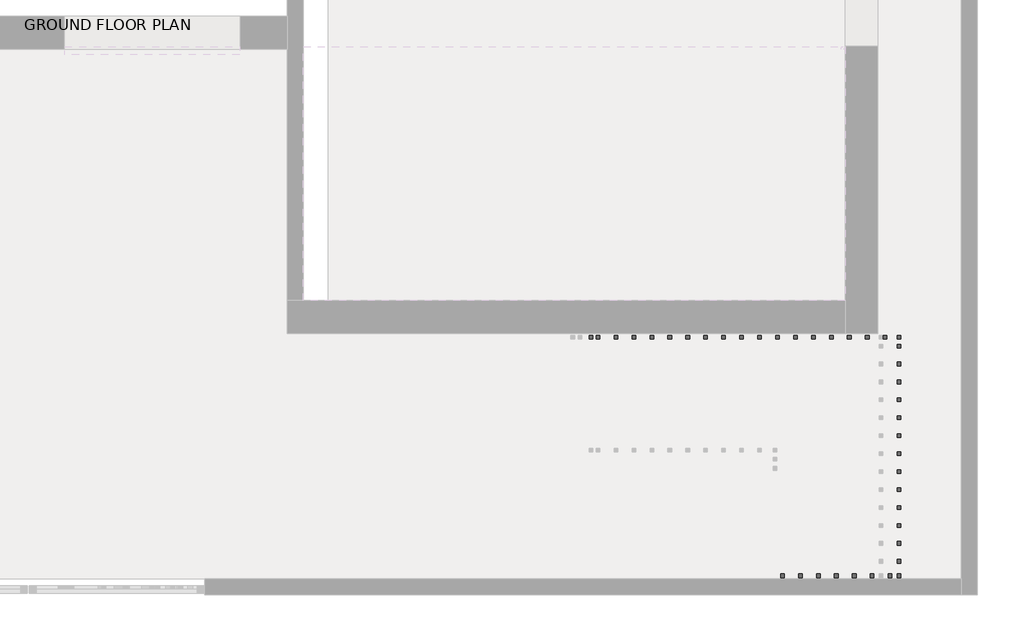
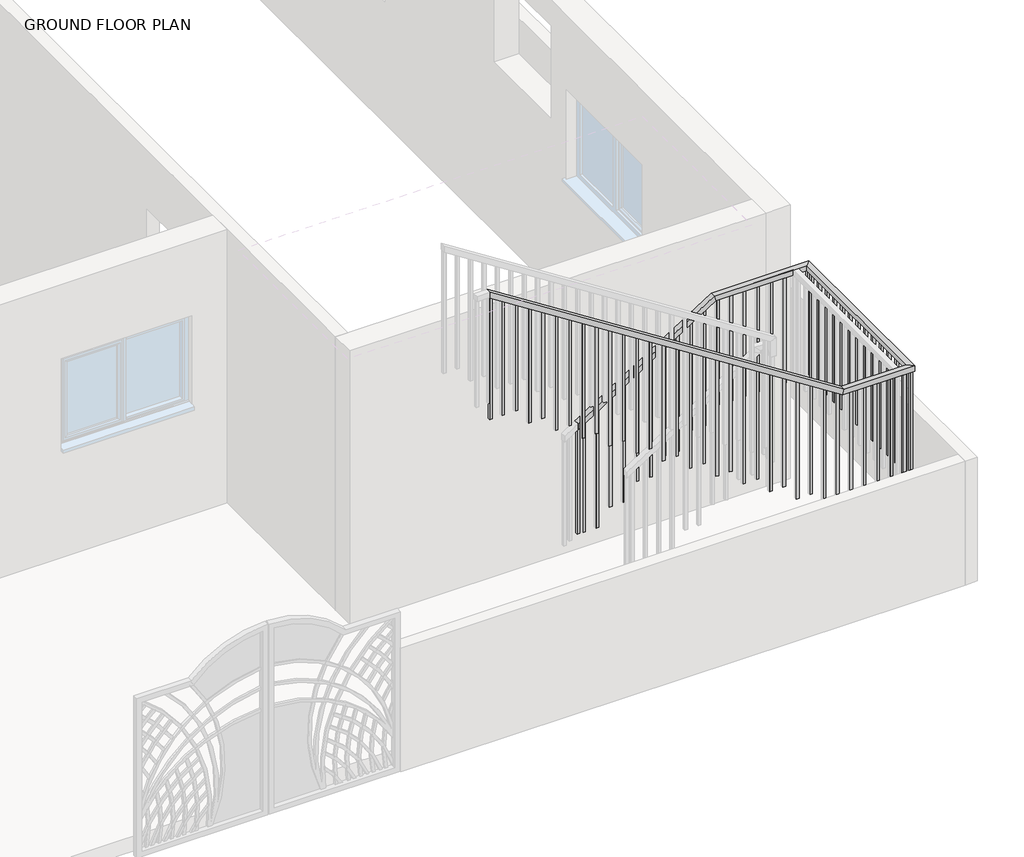
# One storey, part 2 of 23: 2 railings.
"""IFC4 building model written with IfcOpenShell, lengths in millimetres."""

from ifc_helpers import new_model, si_unit, frame, origin, place, context, project, spatial, polyline, outline, extrude, faceted_brep, element, save

model = new_model("IFC4")

# Units and contexts
model_context = context("Model", 3, world=origin())
ifc_project = project(units=[si_unit("LENGTHUNIT", "METRE", prefix="MILLI")], contexts=[model_context])

# Site, building, storey
site = spatial("IfcSite", under=ifc_project)
building = spatial("IfcBuilding", under=site)
storey = spatial("IfcBuildingStorey", under=building, Name="GROUND FLOOR PLAN", Elevation=487.68)

# Railings
placement = place(None, origin())
element("IfcRailing", 1, ObjectType="1100mm", at=placement, inside=storey, context=model_context, shape_type="SolidModel", body=[
    faceted_brep([(-8680.149573, -10220.0521308, 1912.8), (-8680.149573, -10220.0521308, 1853.4423995), (-8680.149573, -10270.0521308, 1853.4423995), (-8680.149573, -10270.0521308, 1912.8), (-7409.7306254, -10220.0521308, 2725.6), (-7395.1045513, -10220.0521308, 2675.6), (-7395.1045513, -10270.0521308, 2675.6), (-7409.7306254, -10270.0521308, 2725.6), (-6495.8132565, -10220.0521308, 2725.6), (-6495.8132565, -10220.0521308, 2675.6), (-6545.8132565, -10270.0521308, 2675.6), (-6545.8132565, -10270.0521308, 2725.6), (-6495.8132565, -11933.6860066, 2725.6), (-6495.8132565, -11933.6860066, 2675.6), (-6545.8132565, -11883.6860066, 2675.6), (-6545.8132565, -11883.6860066, 2725.6), (-7155.718398, -11933.6860066, 2725.6), (-7170.3479429, -11933.6860066, 2675.6), (-7170.3479429, -11883.6860066, 2675.6), (-7155.718398, -11883.6860066, 2725.6), (-10457.8773536, -11933.6860066, 4838.88), (-10457.8773536, -11883.6860066, 4838.88), (-10457.8773536, -11883.6860066, 4779.517542), (-10457.8773536, -11933.6860066, 4779.517542)], [[[0, 1, 2, 3]], [[1, 0, 4, 5]], [[2, 1, 5, 6]], [[3, 2, 6, 7]], [[0, 3, 7, 4]], [[5, 4, 8, 9]], [[6, 5, 9, 10]], [[7, 6, 10, 11]], [[4, 7, 11, 8]], [[9, 8, 12, 13]], [[10, 9, 13, 14]], [[11, 10, 14, 15]], [[8, 11, 15, 12]], [[13, 12, 16, 17]], [[14, 13, 17, 18]], [[15, 14, 18, 19]], [[12, 15, 19, 16]], [[20, 21, 22, 23]], [[17, 16, 20, 23]], [[18, 17, 23, 22]], [[19, 18, 22, 21]], [[16, 19, 21, 20]]]),
    extrude(outline(polyline([(4691.8007425, -10320.8132565), (4707.7999723, -10345.8132565), (3576.32, -10345.8132565), (3576.32, -10320.8132565), (4691.8007425, -10320.8132565)])), frame((0.0, -11921.1860066, 0.0), z_axis=(0.0, 1.0, 0.0), x_axis=(0.0, 0.0, 1.0)), (0.0, 0.0, 1.0), 25.0),
    extrude(outline(polyline([(4611.8045935, -10195.8132565), (4627.8038233, -10220.8132565), (3576.32, -10220.8132565), (3576.32, -10195.8132565), (4611.8045935, -10195.8132565)])), frame((0.0, -11921.1860066, 0.0), z_axis=(0.0, 1.0, 0.0), x_axis=(0.0, 0.0, 1.0)), (0.0, 0.0, 1.0), 25.0),
    extrude(outline(polyline([(4531.8084444, -10070.8132565), (4547.8076742, -10095.8132565), (3413.76, -10095.8132565), (3413.76, -10070.8132565), (4531.8084444, -10070.8132565)])), frame((0.0, -11921.1860066, 0.0), z_axis=(0.0, 1.0, 0.0), x_axis=(0.0, 0.0, 1.0)), (0.0, 0.0, 1.0), 25.0),
    extrude(outline(polyline([(4451.8122954, -9945.8132565), (4467.8115252, -9970.8132565), (3413.76, -9970.8132565), (3413.76, -9945.8132565), (4451.8122954, -9945.8132565)])), frame((0.0, -11921.1860066, 0.0), z_axis=(0.0, 1.0, 0.0), x_axis=(0.0, 0.0, 1.0)), (0.0, 0.0, 1.0), 25.0),
    extrude(outline(polyline([(4371.8161463, -9820.8132565), (4387.8153761, -9845.8132565), (3251.2, -9845.8132565), (3251.2, -9820.8132565), (4371.8161463, -9820.8132565)])), frame((0.0, -11921.1860066, 0.0), z_axis=(0.0, 1.0, 0.0), x_axis=(0.0, 0.0, 1.0)), (0.0, 0.0, 1.0), 25.0),
    extrude(outline(polyline([(4291.8423995, -9695.8132565), (4307.8371231, -9720.8132565), (3251.2, -9720.8132565), (3251.2, -9695.8132565), (4291.8423995, -9695.8132565)])), frame((0.0, -11921.1860066, 0.0), z_axis=(0.0, 1.0, 0.0), x_axis=(0.0, 0.0, 1.0)), (0.0, 0.0, 1.0), 25.0),
    extrude(outline(polyline([(4211.8238482, -9570.8132565), (4227.823078, -9595.8132565), (3088.64, -9595.8132565), (3088.64, -9570.8132565), (4211.8238482, -9570.8132565)])), frame((0.0, -11921.1860066, 0.0), z_axis=(0.0, 1.0, 0.0), x_axis=(0.0, 0.0, 1.0)), (0.0, 0.0, 1.0), 25.0),
    extrude(outline(polyline([(4131.8276992, -9445.8132565), (4147.826929, -9470.8132565), (3088.64, -9470.8132565), (3088.64, -9445.8132565), (4131.8276992, -9445.8132565)])), frame((0.0, -11921.1860066, 0.0), z_axis=(0.0, 1.0, 0.0), x_axis=(0.0, 0.0, 1.0)), (0.0, 0.0, 1.0), 25.0),
    extrude(outline(polyline([(4051.8315501, -9320.8132565), (4067.8307799, -9345.8132565), (2926.08, -9345.8132565), (2926.08, -9320.8132565), (4051.8315501, -9320.8132565)])), frame((0.0, -11921.1860066, 0.0), z_axis=(0.0, 1.0, 0.0), x_axis=(0.0, 0.0, 1.0)), (0.0, 0.0, 1.0), 25.0),
    extrude(outline(polyline([(3971.835401, -9195.8132565), (3987.8346309, -9220.8132565), (2926.08, -9220.8132565), (2926.08, -9195.8132565), (3971.835401, -9195.8132565)])), frame((0.0, -11921.1860066, 0.0), z_axis=(0.0, 1.0, 0.0), x_axis=(0.0, 0.0, 1.0)), (0.0, 0.0, 1.0), 25.0),
    extrude(outline(polyline([(3891.839252, -9070.8132565), (3907.8384818, -9095.8132565), (2763.52, -9095.8132565), (2763.52, -9070.8132565), (3891.839252, -9070.8132565)])), frame((0.0, -11921.1860066, 0.0), z_axis=(0.0, 1.0, 0.0), x_axis=(0.0, 0.0, 1.0)), (0.0, 0.0, 1.0), 25.0),
    extrude(outline(polyline([(3811.8431029, -8945.8132565), (3827.8423328, -8970.8132565), (2763.52, -8970.8132565), (2763.52, -8945.8132565), (3811.8431029, -8945.8132565)])), frame((0.0, -11921.1860066, 0.0), z_axis=(0.0, 1.0, 0.0), x_axis=(0.0, 0.0, 1.0)), (0.0, 0.0, 1.0), 25.0),
    extrude(outline(polyline([(3731.8469539, -8820.8132565), (3747.8461837, -8845.8132565), (2600.96, -8845.8132565), (2600.96, -8820.8132565), (3731.8469539, -8820.8132565)])), frame((0.0, -11921.1860066, 0.0), z_axis=(0.0, 1.0, 0.0), x_axis=(0.0, 0.0, 1.0)), (0.0, 0.0, 1.0), 25.0),
    extrude(outline(polyline([(3651.8508048, -8695.8132565), (3667.8500347, -8720.8132565), (2600.96, -8720.8132565), (2600.96, -8695.8132565), (3651.8508048, -8695.8132565)])), frame((0.0, -11921.1860066, 0.0), z_axis=(0.0, 1.0, 0.0), x_axis=(0.0, 0.0, 1.0)), (0.0, 0.0, 1.0), 25.0),
    extrude(outline(polyline([(3571.8546558, -8570.8132565), (3587.8538856, -8595.8132565), (2438.4, -8595.8132565), (2438.4, -8570.8132565), (3571.8546558, -8570.8132565)])), frame((0.0, -11921.1860066, 0.0), z_axis=(0.0, 1.0, 0.0), x_axis=(0.0, 0.0, 1.0)), (0.0, 0.0, 1.0), 25.0),
    extrude(outline(polyline([(3491.8585067, -8445.8132565), (3507.8577365, -8470.8132565), (2438.4, -8470.8132565), (2438.4, -8445.8132565), (3491.8585067, -8445.8132565)])), frame((0.0, -11921.1860066, 0.0), z_axis=(0.0, 1.0, 0.0), x_axis=(0.0, 0.0, 1.0)), (0.0, 0.0, 1.0), 25.0),
    extrude(outline(polyline([(3411.8623577, -8320.8132565), (3427.8615875, -8345.8132565), (2275.84, -8345.8132565), (2275.84, -8320.8132565), (3411.8623577, -8320.8132565)])), frame((0.0, -11921.1860066, 0.0), z_axis=(0.0, 1.0, 0.0), x_axis=(0.0, 0.0, 1.0)), (0.0, 0.0, 1.0), 25.0),
    extrude(outline(polyline([(3331.8662086, -8195.8132565), (3347.8654384, -8220.8132565), (2275.84, -8220.8132565), (2275.84, -8195.8132565), (3331.8662086, -8195.8132565)])), frame((0.0, -11921.1860066, 0.0), z_axis=(0.0, 1.0, 0.0), x_axis=(0.0, 0.0, 1.0)), (0.0, 0.0, 1.0), 25.0),
    extrude(outline(polyline([(3251.8700596, -8070.8132565), (3267.8692894, -8095.8132565), (2113.28, -8095.8132565), (2113.28, -8070.8132565), (3251.8700596, -8070.8132565)])), frame((0.0, -11921.1860066, 0.0), z_axis=(0.0, 1.0, 0.0), x_axis=(0.0, 0.0, 1.0)), (0.0, 0.0, 1.0), 25.0),
    extrude(outline(polyline([(3171.8739105, -7945.8132565), (3187.8731403, -7970.8132565), (2113.28, -7970.8132565), (2113.28, -7945.8132565), (3171.8739105, -7945.8132565)])), frame((0.0, -11921.1860066, 0.0), z_axis=(0.0, 1.0, 0.0), x_axis=(0.0, 0.0, 1.0)), (0.0, 0.0, 1.0), 25.0),
    extrude(outline(polyline([(3091.8777615, -7820.8132565), (3107.8769913, -7845.8132565), (1950.72, -7845.8132565), (1950.72, -7820.8132565), (3091.8777615, -7820.8132565)])), frame((0.0, -11921.1860066, 0.0), z_axis=(0.0, 1.0, 0.0), x_axis=(0.0, 0.0, 1.0)), (0.0, 0.0, 1.0), 25.0),
    extrude(outline(polyline([(3011.8816124, -7695.8132565), (3027.8808422, -7720.8132565), (1950.72, -7720.8132565), (1950.72, -7695.8132565), (3011.8816124, -7695.8132565)])), frame((0.0, -11921.1860066, 0.0), z_axis=(0.0, 1.0, 0.0), x_axis=(0.0, 0.0, 1.0)), (0.0, 0.0, 1.0), 25.0),
    extrude(outline(polyline([(2931.8854634, -7570.8132565), (2947.8846932, -7595.8132565), (1788.16, -7595.8132565), (1788.16, -7570.8132565), (2931.8854634, -7570.8132565)])), frame((0.0, -11921.1860066, 0.0), z_axis=(0.0, 1.0, 0.0), x_axis=(0.0, 0.0, 1.0)), (0.0, 0.0, 1.0), 25.0),
    extrude(outline(polyline([(2851.8893143, -7445.8132565), (2867.8885441, -7470.8132565), (1788.16, -7470.8132565), (1788.16, -7445.8132565), (2851.8893143, -7445.8132565)])), frame((0.0, -11921.1860066, 0.0), z_axis=(0.0, 1.0, 0.0), x_axis=(0.0, 0.0, 1.0)), (0.0, 0.0, 1.0), 25.0),
    extrude(outline(polyline([(2771.8931653, -7320.8132565), (2787.8923951, -7345.8132565), (1625.6, -7345.8132565), (1625.6, -7320.8132565), (2771.8931653, -7320.8132565)])), frame((0.0, -11921.1860066, 0.0), z_axis=(0.0, 1.0, 0.0), x_axis=(0.0, 0.0, 1.0)), (0.0, 0.0, 1.0), 25.0),
    extrude(outline(polyline([(2691.8970162, -7195.8132565), (2707.896246, -7220.8132565), (1625.6, -7220.8132565), (1625.6, -7195.8132565), (2691.8970162, -7195.8132565)])), frame((0.0, -11921.1860066, 0.0), z_axis=(0.0, 1.0, 0.0), x_axis=(0.0, 0.0, 1.0)), (0.0, 0.0, 1.0), 25.0),
    extrude(outline(polyline([(-7070.8132565, -11921.1860066), (-7095.8132565, -11921.1860066), (-7095.8132565, -11896.1860066), (-7070.8132565, -11896.1860066), (-7070.8132565, -11921.1860066)])), frame((0.0, 0.0, 1625.6), z_axis=(0.0, 0.0, 1.0), x_axis=(1.0, 0.0, 0.0)), (0.0, 0.0, 1.0), 1050.0),
    extrude(outline(polyline([(-6945.8132565, -11921.1860066), (-6970.8132565, -11921.1860066), (-6970.8132565, -11896.1860066), (-6945.8132565, -11896.1860066), (-6945.8132565, -11921.1860066)])), frame((0.0, 0.0, 1625.6), z_axis=(0.0, 0.0, 1.0), x_axis=(1.0, 0.0, 0.0)), (0.0, 0.0, 1.0), 1050.0),
    extrude(outline(polyline([(-6820.8132565, -11921.1860066), (-6845.8132565, -11921.1860066), (-6845.8132565, -11896.1860066), (-6820.8132565, -11896.1860066), (-6820.8132565, -11921.1860066)])), frame((0.0, 0.0, 1625.6), z_axis=(0.0, 0.0, 1.0), x_axis=(1.0, 0.0, 0.0)), (0.0, 0.0, 1.0), 1050.0),
    extrude(outline(polyline([(-6695.8132565, -11921.1860066), (-6720.8132565, -11921.1860066), (-6720.8132565, -11896.1860066), (-6695.8132565, -11896.1860066), (-6695.8132565, -11921.1860066)])), frame((0.0, 0.0, 1625.6), z_axis=(0.0, 0.0, 1.0), x_axis=(1.0, 0.0, 0.0)), (0.0, 0.0, 1.0), 1050.0),
    extrude(outline(polyline([(-6570.8132565, -11921.1860066), (-6595.8132565, -11921.1860066), (-6595.8132565, -11896.1860066), (-6570.8132565, -11896.1860066), (-6570.8132565, -11921.1860066)])), frame((0.0, 0.0, 1625.6), z_axis=(0.0, 0.0, 1.0), x_axis=(1.0, 0.0, 0.0)), (0.0, 0.0, 1.0), 1050.0),
    extrude(outline(polyline([(-6508.3132565, -11795.0521308), (-6508.3132565, -11820.0521308), (-6533.3132565, -11820.0521308), (-6533.3132565, -11795.0521308), (-6508.3132565, -11795.0521308)])), frame((0.0, 0.0, 1625.6), z_axis=(0.0, 0.0, 1.0), x_axis=(1.0, 0.0, 0.0)), (0.0, 0.0, 1.0), 1050.0),
    extrude(outline(polyline([(-6508.3132565, -11670.0521308), (-6508.3132565, -11695.0521308), (-6533.3132565, -11695.0521308), (-6533.3132565, -11670.0521308), (-6508.3132565, -11670.0521308)])), frame((0.0, 0.0, 1625.6), z_axis=(0.0, 0.0, 1.0), x_axis=(1.0, 0.0, 0.0)), (0.0, 0.0, 1.0), 1050.0),
    extrude(outline(polyline([(-6508.3132565, -11545.0521308), (-6508.3132565, -11570.0521308), (-6533.3132565, -11570.0521308), (-6533.3132565, -11545.0521308), (-6508.3132565, -11545.0521308)])), frame((0.0, 0.0, 1625.6), z_axis=(0.0, 0.0, 1.0), x_axis=(1.0, 0.0, 0.0)), (0.0, 0.0, 1.0), 1050.0),
    extrude(outline(polyline([(-6508.3132565, -11420.0521308), (-6508.3132565, -11445.0521308), (-6533.3132565, -11445.0521308), (-6533.3132565, -11420.0521308), (-6508.3132565, -11420.0521308)])), frame((0.0, 0.0, 1625.6), z_axis=(0.0, 0.0, 1.0), x_axis=(1.0, 0.0, 0.0)), (0.0, 0.0, 1.0), 1050.0),
    extrude(outline(polyline([(-6508.3132565, -11295.0521308), (-6508.3132565, -11320.0521308), (-6533.3132565, -11320.0521308), (-6533.3132565, -11295.0521308), (-6508.3132565, -11295.0521308)])), frame((0.0, 0.0, 1625.6), z_axis=(0.0, 0.0, 1.0), x_axis=(1.0, 0.0, 0.0)), (0.0, 0.0, 1.0), 1050.0),
    extrude(outline(polyline([(-6508.3132565, -11170.0521308), (-6508.3132565, -11195.0521308), (-6533.3132565, -11195.0521308), (-6533.3132565, -11170.0521308), (-6508.3132565, -11170.0521308)])), frame((0.0, 0.0, 1625.6), z_axis=(0.0, 0.0, 1.0), x_axis=(1.0, 0.0, 0.0)), (0.0, 0.0, 1.0), 1050.0),
    extrude(outline(polyline([(-6508.3132565, -11045.0521308), (-6508.3132565, -11070.0521308), (-6533.3132565, -11070.0521308), (-6533.3132565, -11045.0521308), (-6508.3132565, -11045.0521308)])), frame((0.0, 0.0, 1625.6), z_axis=(0.0, 0.0, 1.0), x_axis=(1.0, 0.0, 0.0)), (0.0, 0.0, 1.0), 1050.0),
    extrude(outline(polyline([(-6508.3132565, -10920.0521308), (-6508.3132565, -10945.0521308), (-6533.3132565, -10945.0521308), (-6533.3132565, -10920.0521308), (-6508.3132565, -10920.0521308)])), frame((0.0, 0.0, 1625.6), z_axis=(0.0, 0.0, 1.0), x_axis=(1.0, 0.0, 0.0)), (0.0, 0.0, 1.0), 1050.0),
    extrude(outline(polyline([(-6508.3132565, -10795.0521308), (-6508.3132565, -10820.0521308), (-6533.3132565, -10820.0521308), (-6533.3132565, -10795.0521308), (-6508.3132565, -10795.0521308)])), frame((0.0, 0.0, 1625.6), z_axis=(0.0, 0.0, 1.0), x_axis=(1.0, 0.0, 0.0)), (0.0, 0.0, 1.0), 1050.0),
    extrude(outline(polyline([(-6508.3132565, -10670.0521308), (-6508.3132565, -10695.0521308), (-6533.3132565, -10695.0521308), (-6533.3132565, -10670.0521308), (-6508.3132565, -10670.0521308)])), frame((0.0, 0.0, 1625.6), z_axis=(0.0, 0.0, 1.0), x_axis=(1.0, 0.0, 0.0)), (0.0, 0.0, 1.0), 1050.0),
    extrude(outline(polyline([(-6508.3132565, -10545.0521308), (-6508.3132565, -10570.0521308), (-6533.3132565, -10570.0521308), (-6533.3132565, -10545.0521308), (-6508.3132565, -10545.0521308)])), frame((0.0, 0.0, 1625.6), z_axis=(0.0, 0.0, 1.0), x_axis=(1.0, 0.0, 0.0)), (0.0, 0.0, 1.0), 1050.0),
    extrude(outline(polyline([(-6508.3132565, -10420.0521308), (-6508.3132565, -10445.0521308), (-6533.3132565, -10445.0521308), (-6533.3132565, -10420.0521308), (-6508.3132565, -10420.0521308)])), frame((0.0, 0.0, 1625.6), z_axis=(0.0, 0.0, 1.0), x_axis=(1.0, 0.0, 0.0)), (0.0, 0.0, 1.0), 1050.0),
    extrude(outline(polyline([(-6508.3132565, -10295.0521308), (-6508.3132565, -10320.0521308), (-6533.3132565, -10320.0521308), (-6533.3132565, -10295.0521308), (-6508.3132565, -10295.0521308)])), frame((0.0, 0.0, 1625.6), z_axis=(0.0, 0.0, 1.0), x_axis=(1.0, 0.0, 0.0)), (0.0, 0.0, 1.0), 1050.0),
    extrude(outline(polyline([(-6630.149573, -10232.5521308), (-6605.149573, -10232.5521308), (-6605.149573, -10257.5521308), (-6630.149573, -10257.5521308), (-6630.149573, -10232.5521308)])), frame((0.0, 0.0, 1625.6), z_axis=(0.0, 0.0, 1.0), x_axis=(1.0, 0.0, 0.0)), (0.0, 0.0, 1.0), 1050.0),
    extrude(outline(polyline([(-6755.149573, -10232.5521308), (-6730.149573, -10232.5521308), (-6730.149573, -10257.5521308), (-6755.149573, -10257.5521308), (-6755.149573, -10232.5521308)])), frame((0.0, 0.0, 1625.6), z_axis=(0.0, 0.0, 1.0), x_axis=(1.0, 0.0, 0.0)), (0.0, 0.0, 1.0), 1050.0),
    extrude(outline(polyline([(-6880.149573, -10232.5521308), (-6855.149573, -10232.5521308), (-6855.149573, -10257.5521308), (-6880.149573, -10257.5521308), (-6880.149573, -10232.5521308)])), frame((0.0, 0.0, 1625.6), z_axis=(0.0, 0.0, 1.0), x_axis=(1.0, 0.0, 0.0)), (0.0, 0.0, 1.0), 1050.0),
    extrude(outline(polyline([(-7005.149573, -10232.5521308), (-6980.149573, -10232.5521308), (-6980.149573, -10257.5521308), (-7005.149573, -10257.5521308), (-7005.149573, -10232.5521308)])), frame((0.0, 0.0, 1625.6), z_axis=(0.0, 0.0, 1.0), x_axis=(1.0, 0.0, 0.0)), (0.0, 0.0, 1.0), 1050.0),
    extrude(outline(polyline([(-7130.149573, -10232.5521308), (-7105.149573, -10232.5521308), (-7105.149573, -10257.5521308), (-7130.149573, -10257.5521308), (-7130.149573, -10232.5521308)])), frame((0.0, 0.0, 1625.6), z_axis=(0.0, 0.0, 1.0), x_axis=(1.0, 0.0, 0.0)), (0.0, 0.0, 1.0), 1050.0),
    extrude(outline(polyline([(-7255.149573, -10232.5521308), (-7230.149573, -10232.5521308), (-7230.149573, -10257.5521308), (-7255.149573, -10257.5521308), (-7255.149573, -10232.5521308)])), frame((0.0, 0.0, 1625.6), z_axis=(0.0, 0.0, 1.0), x_axis=(1.0, 0.0, 0.0)), (0.0, 0.0, 1.0), 1050.0),
    extrude(outline(polyline([(-7380.149573, -10232.5521308), (-7355.149573, -10232.5521308), (-7355.149573, -10257.5521308), (-7380.149573, -10257.5521308), (-7380.149573, -10232.5521308)])), frame((0.0, 0.0, 1625.6), z_axis=(0.0, 0.0, 1.0), x_axis=(1.0, 0.0, 0.0)), (0.0, 0.0, 1.0), 1050.0),
    extrude(outline(polyline([(1463.04, -7505.149573), (1463.04, -7480.149573), (2621.1891352, -7480.149573), (2605.1944115, -7505.149573), (1463.04, -7505.149573)])), frame((0.0, -10257.5521308, 0.0), z_axis=(0.0, 1.0, 0.0), x_axis=(0.0, 0.0, 1.0)), (0.0, 0.0, 1.0), 25.0),
    extrude(outline(polyline([(1463.04, -7630.149573), (1463.04, -7605.149573), (2541.2155169, -7605.149573), (2525.2207932, -7630.149573), (1463.04, -7630.149573)])), frame((0.0, -10257.5521308, 0.0), z_axis=(0.0, 1.0, 0.0), x_axis=(0.0, 0.0, 1.0)), (0.0, 0.0, 1.0), 25.0),
    extrude(outline(polyline([(1300.48, -7755.149573), (1300.48, -7730.149573), (2461.2418986, -7730.149573), (2445.2471749, -7755.149573), (1300.48, -7755.149573)])), frame((0.0, -10257.5521308, 0.0), z_axis=(0.0, 1.0, 0.0), x_axis=(0.0, 0.0, 1.0)), (0.0, 0.0, 1.0), 25.0),
    extrude(outline(polyline([(1300.48, -7880.149573), (1300.48, -7855.149573), (2381.2682803, -7855.149573), (2365.2735566, -7880.149573), (1300.48, -7880.149573)])), frame((0.0, -10257.5521308, 0.0), z_axis=(0.0, 1.0, 0.0), x_axis=(0.0, 0.0, 1.0)), (0.0, 0.0, 1.0), 25.0),
    extrude(outline(polyline([(1137.92, -8005.149573), (1137.92, -7980.149573), (2301.294662, -7980.149573), (2285.2999383, -8005.149573), (1137.92, -8005.149573)])), frame((0.0, -10257.5521308, 0.0), z_axis=(0.0, 1.0, 0.0), x_axis=(0.0, 0.0, 1.0)), (0.0, 0.0, 1.0), 25.0),
    extrude(outline(polyline([(1137.92, -8130.149573), (1137.92, -8105.149573), (2221.3210437, -8105.149573), (2205.32632, -8130.149573), (1137.92, -8130.149573)])), frame((0.0, -10257.5521308, 0.0), z_axis=(0.0, 1.0, 0.0), x_axis=(0.0, 0.0, 1.0)), (0.0, 0.0, 1.0), 25.0),
    extrude(outline(polyline([(975.36, -8255.149573), (975.36, -8230.149573), (2141.3474254, -8230.149573), (2125.3527017, -8255.149573), (975.36, -8255.149573)])), frame((0.0, -10257.5521308, 0.0), z_axis=(0.0, 1.0, 0.0), x_axis=(0.0, 0.0, 1.0)), (0.0, 0.0, 1.0), 25.0),
    extrude(outline(polyline([(975.36, -8380.149573), (975.36, -8355.149573), (2061.3738071, -8355.149573), (2045.3790834, -8380.149573), (975.36, -8380.149573)])), frame((0.0, -10257.5521308, 0.0), z_axis=(0.0, 1.0, 0.0), x_axis=(0.0, 0.0, 1.0)), (0.0, 0.0, 1.0), 25.0),
    extrude(outline(polyline([(812.8, -8505.149573), (812.8, -8480.149573), (1981.4001888, -8480.149573), (1965.4054651, -8505.149573), (812.8, -8505.149573)])), frame((0.0, -10257.5521308, 0.0), z_axis=(0.0, 1.0, 0.0), x_axis=(0.0, 0.0, 1.0)), (0.0, 0.0, 1.0), 25.0),
    extrude(outline(polyline([(812.8, -8630.149573), (812.8, -8605.149573), (1901.4265705, -8605.149573), (1885.4318468, -8630.149573), (812.8, -8630.149573)])), frame((0.0, -10257.5521308, 0.0), z_axis=(0.0, 1.0, 0.0), x_axis=(0.0, 0.0, 1.0)), (0.0, 0.0, 1.0), 25.0),
    extrude(outline(polyline([(-6508.3132565, -11896.1860066), (-6508.3132565, -11921.1860066), (-6533.3132565, -11921.1860066), (-6533.3132565, -11896.1860066), (-6508.3132565, -11896.1860066)])), frame((0.0, 0.0, 1625.6), z_axis=(0.0, 0.0, 1.0), x_axis=(1.0, 0.0, 0.0)), (0.0, 0.0, 1.0), 1050.0),
    extrude(outline(polyline([(-6533.3132565, -10232.5521308), (-6508.3132565, -10232.5521308), (-6508.3132565, -10257.5521308), (-6533.3132565, -10257.5521308), (-6533.3132565, -10232.5521308)])), frame((0.0, 0.0, 1625.6), z_axis=(0.0, 0.0, 1.0), x_axis=(1.0, 0.0, 0.0)), (0.0, 0.0, 1.0), 1050.0),
    extrude(outline(polyline([(4763.5183122, -10432.8773536), (4779.517542, -10457.8773536), (3576.32, -10457.8773536), (3576.32, -10432.8773536), (4763.5183122, -10432.8773536)])), frame((0.0, -11921.1860066, 0.0), z_axis=(0.0, 1.0, 0.0), x_axis=(0.0, 0.0, 1.0)), (0.0, 0.0, 1.0), 25.0),
    extrude(outline(polyline([(812.8, -8680.149573), (812.8, -8655.149573), (1869.4371231, -8655.149573), (1853.4423995, -8680.149573), (812.8, -8680.149573)])), frame((0.0, -10257.5521308, 0.0), z_axis=(0.0, 1.0, 0.0), x_axis=(0.0, 0.0, 1.0)), (0.0, 0.0, 1.0), 25.0),
])
element("IfcRailing", 2, ObjectType="1100mm", at=placement, inside=storey, context=model_context, shape_type="SolidModel", body=[
    faceted_brep([(-8680.149573, -10220.0521308, 1912.8), (-8680.149573, -10220.0521308, 1853.4423995), (-8680.149573, -10270.0521308, 1853.4423995), (-8680.149573, -10270.0521308, 1912.8), (-7409.7306254, -10220.0521308, 2725.6), (-7395.1045513, -10220.0521308, 2675.6), (-7395.1045513, -10270.0521308, 2675.6), (-7409.7306254, -10270.0521308, 2725.6), (-6495.8132565, -10220.0521308, 2725.6), (-6495.8132565, -10220.0521308, 2675.6), (-6545.8132565, -10270.0521308, 2675.6), (-6545.8132565, -10270.0521308, 2725.6), (-6495.8132565, -11933.6860066, 2725.6), (-6495.8132565, -11933.6860066, 2675.6), (-6545.8132565, -11883.6860066, 2675.6), (-6545.8132565, -11883.6860066, 2725.6), (-7155.718398, -11933.6860066, 2725.6), (-7170.3479429, -11933.6860066, 2675.6), (-7170.3479429, -11883.6860066, 2675.6), (-7155.718398, -11883.6860066, 2725.6), (-10457.8773536, -11933.6860066, 4838.88), (-10457.8773536, -11883.6860066, 4838.88), (-10457.8773536, -11883.6860066, 4779.517542), (-10457.8773536, -11933.6860066, 4779.517542)], [[[0, 1, 2, 3]], [[1, 0, 4, 5]], [[2, 1, 5, 6]], [[3, 2, 6, 7]], [[0, 3, 7, 4]], [[5, 4, 8, 9]], [[6, 5, 9, 10]], [[7, 6, 10, 11]], [[4, 7, 11, 8]], [[9, 8, 12, 13]], [[10, 9, 13, 14]], [[11, 10, 14, 15]], [[8, 11, 15, 12]], [[13, 12, 16, 17]], [[14, 13, 17, 18]], [[15, 14, 18, 19]], [[12, 15, 19, 16]], [[20, 21, 22, 23]], [[17, 16, 20, 23]], [[18, 17, 23, 22]], [[19, 18, 22, 21]], [[16, 19, 21, 20]]]),
    extrude(outline(polyline([(4691.8007425, -10320.8132565), (4707.7999723, -10345.8132565), (3576.32, -10345.8132565), (3576.32, -10320.8132565), (4691.8007425, -10320.8132565)])), frame((0.0, -11921.1860066, 0.0), z_axis=(0.0, 1.0, 0.0), x_axis=(0.0, 0.0, 1.0)), (0.0, 0.0, 1.0), 25.0),
    extrude(outline(polyline([(4611.8045935, -10195.8132565), (4627.8038233, -10220.8132565), (3576.32, -10220.8132565), (3576.32, -10195.8132565), (4611.8045935, -10195.8132565)])), frame((0.0, -11921.1860066, 0.0), z_axis=(0.0, 1.0, 0.0), x_axis=(0.0, 0.0, 1.0)), (0.0, 0.0, 1.0), 25.0),
    extrude(outline(polyline([(4531.8084444, -10070.8132565), (4547.8076742, -10095.8132565), (3413.76, -10095.8132565), (3413.76, -10070.8132565), (4531.8084444, -10070.8132565)])), frame((0.0, -11921.1860066, 0.0), z_axis=(0.0, 1.0, 0.0), x_axis=(0.0, 0.0, 1.0)), (0.0, 0.0, 1.0), 25.0),
    extrude(outline(polyline([(4451.8122954, -9945.8132565), (4467.8115252, -9970.8132565), (3413.76, -9970.8132565), (3413.76, -9945.8132565), (4451.8122954, -9945.8132565)])), frame((0.0, -11921.1860066, 0.0), z_axis=(0.0, 1.0, 0.0), x_axis=(0.0, 0.0, 1.0)), (0.0, 0.0, 1.0), 25.0),
    extrude(outline(polyline([(4371.8161463, -9820.8132565), (4387.8153761, -9845.8132565), (3251.2, -9845.8132565), (3251.2, -9820.8132565), (4371.8161463, -9820.8132565)])), frame((0.0, -11921.1860066, 0.0), z_axis=(0.0, 1.0, 0.0), x_axis=(0.0, 0.0, 1.0)), (0.0, 0.0, 1.0), 25.0),
    extrude(outline(polyline([(4291.8423995, -9695.8132565), (4307.8371231, -9720.8132565), (3251.2, -9720.8132565), (3251.2, -9695.8132565), (4291.8423995, -9695.8132565)])), frame((0.0, -11921.1860066, 0.0), z_axis=(0.0, 1.0, 0.0), x_axis=(0.0, 0.0, 1.0)), (0.0, 0.0, 1.0), 25.0),
    extrude(outline(polyline([(4211.8238482, -9570.8132565), (4227.823078, -9595.8132565), (3088.64, -9595.8132565), (3088.64, -9570.8132565), (4211.8238482, -9570.8132565)])), frame((0.0, -11921.1860066, 0.0), z_axis=(0.0, 1.0, 0.0), x_axis=(0.0, 0.0, 1.0)), (0.0, 0.0, 1.0), 25.0),
    extrude(outline(polyline([(4131.8276992, -9445.8132565), (4147.826929, -9470.8132565), (3088.64, -9470.8132565), (3088.64, -9445.8132565), (4131.8276992, -9445.8132565)])), frame((0.0, -11921.1860066, 0.0), z_axis=(0.0, 1.0, 0.0), x_axis=(0.0, 0.0, 1.0)), (0.0, 0.0, 1.0), 25.0),
    extrude(outline(polyline([(4051.8315501, -9320.8132565), (4067.8307799, -9345.8132565), (2926.08, -9345.8132565), (2926.08, -9320.8132565), (4051.8315501, -9320.8132565)])), frame((0.0, -11921.1860066, 0.0), z_axis=(0.0, 1.0, 0.0), x_axis=(0.0, 0.0, 1.0)), (0.0, 0.0, 1.0), 25.0),
    extrude(outline(polyline([(3971.835401, -9195.8132565), (3987.8346309, -9220.8132565), (2926.08, -9220.8132565), (2926.08, -9195.8132565), (3971.835401, -9195.8132565)])), frame((0.0, -11921.1860066, 0.0), z_axis=(0.0, 1.0, 0.0), x_axis=(0.0, 0.0, 1.0)), (0.0, 0.0, 1.0), 25.0),
    extrude(outline(polyline([(3891.839252, -9070.8132565), (3907.8384818, -9095.8132565), (2763.52, -9095.8132565), (2763.52, -9070.8132565), (3891.839252, -9070.8132565)])), frame((0.0, -11921.1860066, 0.0), z_axis=(0.0, 1.0, 0.0), x_axis=(0.0, 0.0, 1.0)), (0.0, 0.0, 1.0), 25.0),
    extrude(outline(polyline([(3811.8431029, -8945.8132565), (3827.8423328, -8970.8132565), (2763.52, -8970.8132565), (2763.52, -8945.8132565), (3811.8431029, -8945.8132565)])), frame((0.0, -11921.1860066, 0.0), z_axis=(0.0, 1.0, 0.0), x_axis=(0.0, 0.0, 1.0)), (0.0, 0.0, 1.0), 25.0),
    extrude(outline(polyline([(3731.8469539, -8820.8132565), (3747.8461837, -8845.8132565), (2600.96, -8845.8132565), (2600.96, -8820.8132565), (3731.8469539, -8820.8132565)])), frame((0.0, -11921.1860066, 0.0), z_axis=(0.0, 1.0, 0.0), x_axis=(0.0, 0.0, 1.0)), (0.0, 0.0, 1.0), 25.0),
    extrude(outline(polyline([(3651.8508048, -8695.8132565), (3667.8500347, -8720.8132565), (2600.96, -8720.8132565), (2600.96, -8695.8132565), (3651.8508048, -8695.8132565)])), frame((0.0, -11921.1860066, 0.0), z_axis=(0.0, 1.0, 0.0), x_axis=(0.0, 0.0, 1.0)), (0.0, 0.0, 1.0), 25.0),
    extrude(outline(polyline([(3571.8546558, -8570.8132565), (3587.8538856, -8595.8132565), (2438.4, -8595.8132565), (2438.4, -8570.8132565), (3571.8546558, -8570.8132565)])), frame((0.0, -11921.1860066, 0.0), z_axis=(0.0, 1.0, 0.0), x_axis=(0.0, 0.0, 1.0)), (0.0, 0.0, 1.0), 25.0),
    extrude(outline(polyline([(3491.8585067, -8445.8132565), (3507.8577365, -8470.8132565), (2438.4, -8470.8132565), (2438.4, -8445.8132565), (3491.8585067, -8445.8132565)])), frame((0.0, -11921.1860066, 0.0), z_axis=(0.0, 1.0, 0.0), x_axis=(0.0, 0.0, 1.0)), (0.0, 0.0, 1.0), 25.0),
    extrude(outline(polyline([(3411.8623577, -8320.8132565), (3427.8615875, -8345.8132565), (2275.84, -8345.8132565), (2275.84, -8320.8132565), (3411.8623577, -8320.8132565)])), frame((0.0, -11921.1860066, 0.0), z_axis=(0.0, 1.0, 0.0), x_axis=(0.0, 0.0, 1.0)), (0.0, 0.0, 1.0), 25.0),
    extrude(outline(polyline([(3331.8662086, -8195.8132565), (3347.8654384, -8220.8132565), (2275.84, -8220.8132565), (2275.84, -8195.8132565), (3331.8662086, -8195.8132565)])), frame((0.0, -11921.1860066, 0.0), z_axis=(0.0, 1.0, 0.0), x_axis=(0.0, 0.0, 1.0)), (0.0, 0.0, 1.0), 25.0),
    extrude(outline(polyline([(3251.8700596, -8070.8132565), (3267.8692894, -8095.8132565), (2113.28, -8095.8132565), (2113.28, -8070.8132565), (3251.8700596, -8070.8132565)])), frame((0.0, -11921.1860066, 0.0), z_axis=(0.0, 1.0, 0.0), x_axis=(0.0, 0.0, 1.0)), (0.0, 0.0, 1.0), 25.0),
    extrude(outline(polyline([(3171.8739105, -7945.8132565), (3187.8731403, -7970.8132565), (2113.28, -7970.8132565), (2113.28, -7945.8132565), (3171.8739105, -7945.8132565)])), frame((0.0, -11921.1860066, 0.0), z_axis=(0.0, 1.0, 0.0), x_axis=(0.0, 0.0, 1.0)), (0.0, 0.0, 1.0), 25.0),
    extrude(outline(polyline([(3091.8777615, -7820.8132565), (3107.8769913, -7845.8132565), (1950.72, -7845.8132565), (1950.72, -7820.8132565), (3091.8777615, -7820.8132565)])), frame((0.0, -11921.1860066, 0.0), z_axis=(0.0, 1.0, 0.0), x_axis=(0.0, 0.0, 1.0)), (0.0, 0.0, 1.0), 25.0),
    extrude(outline(polyline([(3011.8816124, -7695.8132565), (3027.8808422, -7720.8132565), (1950.72, -7720.8132565), (1950.72, -7695.8132565), (3011.8816124, -7695.8132565)])), frame((0.0, -11921.1860066, 0.0), z_axis=(0.0, 1.0, 0.0), x_axis=(0.0, 0.0, 1.0)), (0.0, 0.0, 1.0), 25.0),
    extrude(outline(polyline([(2931.8854634, -7570.8132565), (2947.8846932, -7595.8132565), (1788.16, -7595.8132565), (1788.16, -7570.8132565), (2931.8854634, -7570.8132565)])), frame((0.0, -11921.1860066, 0.0), z_axis=(0.0, 1.0, 0.0), x_axis=(0.0, 0.0, 1.0)), (0.0, 0.0, 1.0), 25.0),
    extrude(outline(polyline([(2851.8893143, -7445.8132565), (2867.8885441, -7470.8132565), (1788.16, -7470.8132565), (1788.16, -7445.8132565), (2851.8893143, -7445.8132565)])), frame((0.0, -11921.1860066, 0.0), z_axis=(0.0, 1.0, 0.0), x_axis=(0.0, 0.0, 1.0)), (0.0, 0.0, 1.0), 25.0),
    extrude(outline(polyline([(2771.8931653, -7320.8132565), (2787.8923951, -7345.8132565), (1625.6, -7345.8132565), (1625.6, -7320.8132565), (2771.8931653, -7320.8132565)])), frame((0.0, -11921.1860066, 0.0), z_axis=(0.0, 1.0, 0.0), x_axis=(0.0, 0.0, 1.0)), (0.0, 0.0, 1.0), 25.0),
    extrude(outline(polyline([(2691.8970162, -7195.8132565), (2707.896246, -7220.8132565), (1625.6, -7220.8132565), (1625.6, -7195.8132565), (2691.8970162, -7195.8132565)])), frame((0.0, -11921.1860066, 0.0), z_axis=(0.0, 1.0, 0.0), x_axis=(0.0, 0.0, 1.0)), (0.0, 0.0, 1.0), 25.0),
    extrude(outline(polyline([(-7070.8132565, -11921.1860066), (-7095.8132565, -11921.1860066), (-7095.8132565, -11896.1860066), (-7070.8132565, -11896.1860066), (-7070.8132565, -11921.1860066)])), frame((0.0, 0.0, 1625.6), z_axis=(0.0, 0.0, 1.0), x_axis=(1.0, 0.0, 0.0)), (0.0, 0.0, 1.0), 1050.0),
    extrude(outline(polyline([(-6945.8132565, -11921.1860066), (-6970.8132565, -11921.1860066), (-6970.8132565, -11896.1860066), (-6945.8132565, -11896.1860066), (-6945.8132565, -11921.1860066)])), frame((0.0, 0.0, 1625.6), z_axis=(0.0, 0.0, 1.0), x_axis=(1.0, 0.0, 0.0)), (0.0, 0.0, 1.0), 1050.0),
    extrude(outline(polyline([(-6820.8132565, -11921.1860066), (-6845.8132565, -11921.1860066), (-6845.8132565, -11896.1860066), (-6820.8132565, -11896.1860066), (-6820.8132565, -11921.1860066)])), frame((0.0, 0.0, 1625.6), z_axis=(0.0, 0.0, 1.0), x_axis=(1.0, 0.0, 0.0)), (0.0, 0.0, 1.0), 1050.0),
    extrude(outline(polyline([(-6695.8132565, -11921.1860066), (-6720.8132565, -11921.1860066), (-6720.8132565, -11896.1860066), (-6695.8132565, -11896.1860066), (-6695.8132565, -11921.1860066)])), frame((0.0, 0.0, 1625.6), z_axis=(0.0, 0.0, 1.0), x_axis=(1.0, 0.0, 0.0)), (0.0, 0.0, 1.0), 1050.0),
    extrude(outline(polyline([(-6570.8132565, -11921.1860066), (-6595.8132565, -11921.1860066), (-6595.8132565, -11896.1860066), (-6570.8132565, -11896.1860066), (-6570.8132565, -11921.1860066)])), frame((0.0, 0.0, 1625.6), z_axis=(0.0, 0.0, 1.0), x_axis=(1.0, 0.0, 0.0)), (0.0, 0.0, 1.0), 1050.0),
    extrude(outline(polyline([(-6508.3132565, -11795.0521308), (-6508.3132565, -11820.0521308), (-6533.3132565, -11820.0521308), (-6533.3132565, -11795.0521308), (-6508.3132565, -11795.0521308)])), frame((0.0, 0.0, 1625.6), z_axis=(0.0, 0.0, 1.0), x_axis=(1.0, 0.0, 0.0)), (0.0, 0.0, 1.0), 1050.0),
    extrude(outline(polyline([(-6508.3132565, -11670.0521308), (-6508.3132565, -11695.0521308), (-6533.3132565, -11695.0521308), (-6533.3132565, -11670.0521308), (-6508.3132565, -11670.0521308)])), frame((0.0, 0.0, 1625.6), z_axis=(0.0, 0.0, 1.0), x_axis=(1.0, 0.0, 0.0)), (0.0, 0.0, 1.0), 1050.0),
    extrude(outline(polyline([(-6508.3132565, -11545.0521308), (-6508.3132565, -11570.0521308), (-6533.3132565, -11570.0521308), (-6533.3132565, -11545.0521308), (-6508.3132565, -11545.0521308)])), frame((0.0, 0.0, 1625.6), z_axis=(0.0, 0.0, 1.0), x_axis=(1.0, 0.0, 0.0)), (0.0, 0.0, 1.0), 1050.0),
    extrude(outline(polyline([(-6508.3132565, -11420.0521308), (-6508.3132565, -11445.0521308), (-6533.3132565, -11445.0521308), (-6533.3132565, -11420.0521308), (-6508.3132565, -11420.0521308)])), frame((0.0, 0.0, 1625.6), z_axis=(0.0, 0.0, 1.0), x_axis=(1.0, 0.0, 0.0)), (0.0, 0.0, 1.0), 1050.0),
    extrude(outline(polyline([(-6508.3132565, -11295.0521308), (-6508.3132565, -11320.0521308), (-6533.3132565, -11320.0521308), (-6533.3132565, -11295.0521308), (-6508.3132565, -11295.0521308)])), frame((0.0, 0.0, 1625.6), z_axis=(0.0, 0.0, 1.0), x_axis=(1.0, 0.0, 0.0)), (0.0, 0.0, 1.0), 1050.0),
    extrude(outline(polyline([(-6508.3132565, -11170.0521308), (-6508.3132565, -11195.0521308), (-6533.3132565, -11195.0521308), (-6533.3132565, -11170.0521308), (-6508.3132565, -11170.0521308)])), frame((0.0, 0.0, 1625.6), z_axis=(0.0, 0.0, 1.0), x_axis=(1.0, 0.0, 0.0)), (0.0, 0.0, 1.0), 1050.0),
    extrude(outline(polyline([(-6508.3132565, -11045.0521308), (-6508.3132565, -11070.0521308), (-6533.3132565, -11070.0521308), (-6533.3132565, -11045.0521308), (-6508.3132565, -11045.0521308)])), frame((0.0, 0.0, 1625.6), z_axis=(0.0, 0.0, 1.0), x_axis=(1.0, 0.0, 0.0)), (0.0, 0.0, 1.0), 1050.0),
    extrude(outline(polyline([(-6508.3132565, -10920.0521308), (-6508.3132565, -10945.0521308), (-6533.3132565, -10945.0521308), (-6533.3132565, -10920.0521308), (-6508.3132565, -10920.0521308)])), frame((0.0, 0.0, 1625.6), z_axis=(0.0, 0.0, 1.0), x_axis=(1.0, 0.0, 0.0)), (0.0, 0.0, 1.0), 1050.0),
    extrude(outline(polyline([(-6508.3132565, -10795.0521308), (-6508.3132565, -10820.0521308), (-6533.3132565, -10820.0521308), (-6533.3132565, -10795.0521308), (-6508.3132565, -10795.0521308)])), frame((0.0, 0.0, 1625.6), z_axis=(0.0, 0.0, 1.0), x_axis=(1.0, 0.0, 0.0)), (0.0, 0.0, 1.0), 1050.0),
    extrude(outline(polyline([(-6508.3132565, -10670.0521308), (-6508.3132565, -10695.0521308), (-6533.3132565, -10695.0521308), (-6533.3132565, -10670.0521308), (-6508.3132565, -10670.0521308)])), frame((0.0, 0.0, 1625.6), z_axis=(0.0, 0.0, 1.0), x_axis=(1.0, 0.0, 0.0)), (0.0, 0.0, 1.0), 1050.0),
    extrude(outline(polyline([(-6508.3132565, -10545.0521308), (-6508.3132565, -10570.0521308), (-6533.3132565, -10570.0521308), (-6533.3132565, -10545.0521308), (-6508.3132565, -10545.0521308)])), frame((0.0, 0.0, 1625.6), z_axis=(0.0, 0.0, 1.0), x_axis=(1.0, 0.0, 0.0)), (0.0, 0.0, 1.0), 1050.0),
    extrude(outline(polyline([(-6508.3132565, -10420.0521308), (-6508.3132565, -10445.0521308), (-6533.3132565, -10445.0521308), (-6533.3132565, -10420.0521308), (-6508.3132565, -10420.0521308)])), frame((0.0, 0.0, 1625.6), z_axis=(0.0, 0.0, 1.0), x_axis=(1.0, 0.0, 0.0)), (0.0, 0.0, 1.0), 1050.0),
    extrude(outline(polyline([(-6508.3132565, -10295.0521308), (-6508.3132565, -10320.0521308), (-6533.3132565, -10320.0521308), (-6533.3132565, -10295.0521308), (-6508.3132565, -10295.0521308)])), frame((0.0, 0.0, 1625.6), z_axis=(0.0, 0.0, 1.0), x_axis=(1.0, 0.0, 0.0)), (0.0, 0.0, 1.0), 1050.0),
    extrude(outline(polyline([(-6630.149573, -10232.5521308), (-6605.149573, -10232.5521308), (-6605.149573, -10257.5521308), (-6630.149573, -10257.5521308), (-6630.149573, -10232.5521308)])), frame((0.0, 0.0, 1625.6), z_axis=(0.0, 0.0, 1.0), x_axis=(1.0, 0.0, 0.0)), (0.0, 0.0, 1.0), 1050.0),
    extrude(outline(polyline([(-6755.149573, -10232.5521308), (-6730.149573, -10232.5521308), (-6730.149573, -10257.5521308), (-6755.149573, -10257.5521308), (-6755.149573, -10232.5521308)])), frame((0.0, 0.0, 1625.6), z_axis=(0.0, 0.0, 1.0), x_axis=(1.0, 0.0, 0.0)), (0.0, 0.0, 1.0), 1050.0),
    extrude(outline(polyline([(-6880.149573, -10232.5521308), (-6855.149573, -10232.5521308), (-6855.149573, -10257.5521308), (-6880.149573, -10257.5521308), (-6880.149573, -10232.5521308)])), frame((0.0, 0.0, 1625.6), z_axis=(0.0, 0.0, 1.0), x_axis=(1.0, 0.0, 0.0)), (0.0, 0.0, 1.0), 1050.0),
    extrude(outline(polyline([(-7005.149573, -10232.5521308), (-6980.149573, -10232.5521308), (-6980.149573, -10257.5521308), (-7005.149573, -10257.5521308), (-7005.149573, -10232.5521308)])), frame((0.0, 0.0, 1625.6), z_axis=(0.0, 0.0, 1.0), x_axis=(1.0, 0.0, 0.0)), (0.0, 0.0, 1.0), 1050.0),
    extrude(outline(polyline([(-7130.149573, -10232.5521308), (-7105.149573, -10232.5521308), (-7105.149573, -10257.5521308), (-7130.149573, -10257.5521308), (-7130.149573, -10232.5521308)])), frame((0.0, 0.0, 1625.6), z_axis=(0.0, 0.0, 1.0), x_axis=(1.0, 0.0, 0.0)), (0.0, 0.0, 1.0), 1050.0),
    extrude(outline(polyline([(-7255.149573, -10232.5521308), (-7230.149573, -10232.5521308), (-7230.149573, -10257.5521308), (-7255.149573, -10257.5521308), (-7255.149573, -10232.5521308)])), frame((0.0, 0.0, 1625.6), z_axis=(0.0, 0.0, 1.0), x_axis=(1.0, 0.0, 0.0)), (0.0, 0.0, 1.0), 1050.0),
    extrude(outline(polyline([(-7380.149573, -10232.5521308), (-7355.149573, -10232.5521308), (-7355.149573, -10257.5521308), (-7380.149573, -10257.5521308), (-7380.149573, -10232.5521308)])), frame((0.0, 0.0, 1625.6), z_axis=(0.0, 0.0, 1.0), x_axis=(1.0, 0.0, 0.0)), (0.0, 0.0, 1.0), 1050.0),
    extrude(outline(polyline([(1463.04, -7505.149573), (1463.04, -7480.149573), (2621.1891352, -7480.149573), (2605.1944115, -7505.149573), (1463.04, -7505.149573)])), frame((0.0, -10257.5521308, 0.0), z_axis=(0.0, 1.0, 0.0), x_axis=(0.0, 0.0, 1.0)), (0.0, 0.0, 1.0), 25.0),
    extrude(outline(polyline([(1463.04, -7630.149573), (1463.04, -7605.149573), (2541.2155169, -7605.149573), (2525.2207932, -7630.149573), (1463.04, -7630.149573)])), frame((0.0, -10257.5521308, 0.0), z_axis=(0.0, 1.0, 0.0), x_axis=(0.0, 0.0, 1.0)), (0.0, 0.0, 1.0), 25.0),
    extrude(outline(polyline([(1300.48, -7755.149573), (1300.48, -7730.149573), (2461.2418986, -7730.149573), (2445.2471749, -7755.149573), (1300.48, -7755.149573)])), frame((0.0, -10257.5521308, 0.0), z_axis=(0.0, 1.0, 0.0), x_axis=(0.0, 0.0, 1.0)), (0.0, 0.0, 1.0), 25.0),
    extrude(outline(polyline([(1300.48, -7880.149573), (1300.48, -7855.149573), (2381.2682803, -7855.149573), (2365.2735566, -7880.149573), (1300.48, -7880.149573)])), frame((0.0, -10257.5521308, 0.0), z_axis=(0.0, 1.0, 0.0), x_axis=(0.0, 0.0, 1.0)), (0.0, 0.0, 1.0), 25.0),
    extrude(outline(polyline([(1137.92, -8005.149573), (1137.92, -7980.149573), (2301.294662, -7980.149573), (2285.2999383, -8005.149573), (1137.92, -8005.149573)])), frame((0.0, -10257.5521308, 0.0), z_axis=(0.0, 1.0, 0.0), x_axis=(0.0, 0.0, 1.0)), (0.0, 0.0, 1.0), 25.0),
    extrude(outline(polyline([(1137.92, -8130.149573), (1137.92, -8105.149573), (2221.3210437, -8105.149573), (2205.32632, -8130.149573), (1137.92, -8130.149573)])), frame((0.0, -10257.5521308, 0.0), z_axis=(0.0, 1.0, 0.0), x_axis=(0.0, 0.0, 1.0)), (0.0, 0.0, 1.0), 25.0),
    extrude(outline(polyline([(975.36, -8255.149573), (975.36, -8230.149573), (2141.3474254, -8230.149573), (2125.3527017, -8255.149573), (975.36, -8255.149573)])), frame((0.0, -10257.5521308, 0.0), z_axis=(0.0, 1.0, 0.0), x_axis=(0.0, 0.0, 1.0)), (0.0, 0.0, 1.0), 25.0),
    extrude(outline(polyline([(975.36, -8380.149573), (975.36, -8355.149573), (2061.3738071, -8355.149573), (2045.3790834, -8380.149573), (975.36, -8380.149573)])), frame((0.0, -10257.5521308, 0.0), z_axis=(0.0, 1.0, 0.0), x_axis=(0.0, 0.0, 1.0)), (0.0, 0.0, 1.0), 25.0),
    extrude(outline(polyline([(812.8, -8505.149573), (812.8, -8480.149573), (1981.4001888, -8480.149573), (1965.4054651, -8505.149573), (812.8, -8505.149573)])), frame((0.0, -10257.5521308, 0.0), z_axis=(0.0, 1.0, 0.0), x_axis=(0.0, 0.0, 1.0)), (0.0, 0.0, 1.0), 25.0),
    extrude(outline(polyline([(812.8, -8630.149573), (812.8, -8605.149573), (1901.4265705, -8605.149573), (1885.4318468, -8630.149573), (812.8, -8630.149573)])), frame((0.0, -10257.5521308, 0.0), z_axis=(0.0, 1.0, 0.0), x_axis=(0.0, 0.0, 1.0)), (0.0, 0.0, 1.0), 25.0),
    extrude(outline(polyline([(-6508.3132565, -11896.1860066), (-6508.3132565, -11921.1860066), (-6533.3132565, -11921.1860066), (-6533.3132565, -11896.1860066), (-6508.3132565, -11896.1860066)])), frame((0.0, 0.0, 1625.6), z_axis=(0.0, 0.0, 1.0), x_axis=(1.0, 0.0, 0.0)), (0.0, 0.0, 1.0), 1050.0),
    extrude(outline(polyline([(-6533.3132565, -10232.5521308), (-6508.3132565, -10232.5521308), (-6508.3132565, -10257.5521308), (-6533.3132565, -10257.5521308), (-6533.3132565, -10232.5521308)])), frame((0.0, 0.0, 1625.6), z_axis=(0.0, 0.0, 1.0), x_axis=(1.0, 0.0, 0.0)), (0.0, 0.0, 1.0), 1050.0),
    extrude(outline(polyline([(4763.5183122, -10432.8773536), (4779.517542, -10457.8773536), (3576.32, -10457.8773536), (3576.32, -10432.8773536), (4763.5183122, -10432.8773536)])), frame((0.0, -11921.1860066, 0.0), z_axis=(0.0, 1.0, 0.0), x_axis=(0.0, 0.0, 1.0)), (0.0, 0.0, 1.0), 25.0),
    extrude(outline(polyline([(812.8, -8680.149573), (812.8, -8655.149573), (1869.4371231, -8655.149573), (1853.4423995, -8680.149573), (812.8, -8680.149573)])), frame((0.0, -10257.5521308, 0.0), z_axis=(0.0, 1.0, 0.0), x_axis=(0.0, 0.0, 1.0)), (0.0, 0.0, 1.0), 25.0),
])

save(model, "model.ifc")

# Revit data of these elements
# Type "1100mm"
#   built-in parameter 1008612 = 0.019685 (stored number, unit not read)
#   built-in parameter 1008611 = 0.019685 (stored number, unit not read)
#   built-in parameter 1008609 = 0.902231 (stored number, unit not read)
#   built-in parameter 1008604 = 0.19685 (stored number, unit not read)
#   built-in parameter 1008603 = 0.164042 (stored number, unit not read)
#   Railing Height = 3.608924 ft
#   built-in parameter 1008630 = 2
#   built-in parameter 1008610 = 2
#   built-in parameter 1008608 = 1
#   built-in parameter 1008618 = Baluster_Square : 25mm
# Elements 1, 2 (IfcRailing, "1100mm")
#   Phase Created = New Construction
